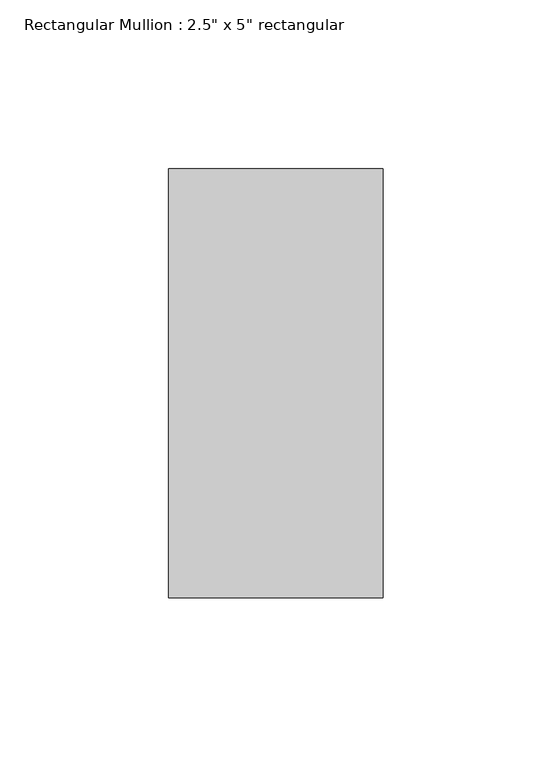
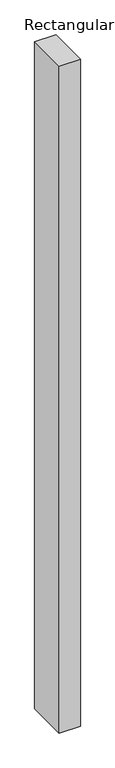
"""IFC4 building model written with IfcOpenShell, lengths in millimetres: member geometry."""

from ifc_helpers import new_model, si_unit, frame, origin, place, context, project, spatial, polyline, outline, extrude, source, transform, mapped, element, save


def member_8f4b05ff(model_context):
    return source(origin(), model_context, "Body", "SweptSolid", [
        extrude(outline(polyline([(0.0, 63.5), (0.0, -63.5), (-63.5, -63.5), (-63.5, 63.5), (0.0, 63.5)])), frame((0.0, 0.0, -2114.55), z_axis=(0.0, 0.0, 1.0), x_axis=(1.0, 0.0, 0.0)), (0.0, 0.0, 1.0), 2114.55),
    ])


if __name__ == "__main__":
    model = new_model("IFC4")
    model_context = context("Model", 3, world=origin())
    ifc_project = project(units=[si_unit("LENGTHUNIT", "METRE", prefix="MILLI")], contexts=[model_context])
    site = spatial("IfcSite", under=ifc_project)
    building = spatial("IfcBuilding", under=site)
    placement = place(None, origin())
    member_shape = member_8f4b05ff(model_context)
    element("IfcMember", 1, ObjectType="Rectangular Mullion : 2.5\" x 5\" rectangular", at=placement, inside=building, context=model_context, shape_type="MappedRepresentation", body=[
        mapped(member_shape, transform((0.0, 0.0, 0.0), x_axis=(1.0, 0.0, 0.0), y_axis=(0.0, 1.0, 0.0), z_axis=(0.0, 0.0, 1.0))),
    ])
    save(model, "model.ifc")

# Revit data of these elements
# Type "Rectangular Mullion : 2.5\" x 5\" rectangular"
#   built-in parameter 1007304 = 0.416667 (stored number, unit not read)
#   built-in parameter 1007301 = 0.104167 (stored number, unit not read)
#   built-in parameter 1007300 = 0.104167 (stored number, unit not read)
# Element 1 (IfcMember, "Rectangular Mullion : 2.5\" x 5\" rectangular")
#   Materials on its faces: "Aluminum"
# Materials
#   "Aluminum": class "Metal", colour RGB 247 247 247, transparency 0, Description = "Aluminum 6061", Cost = 0
